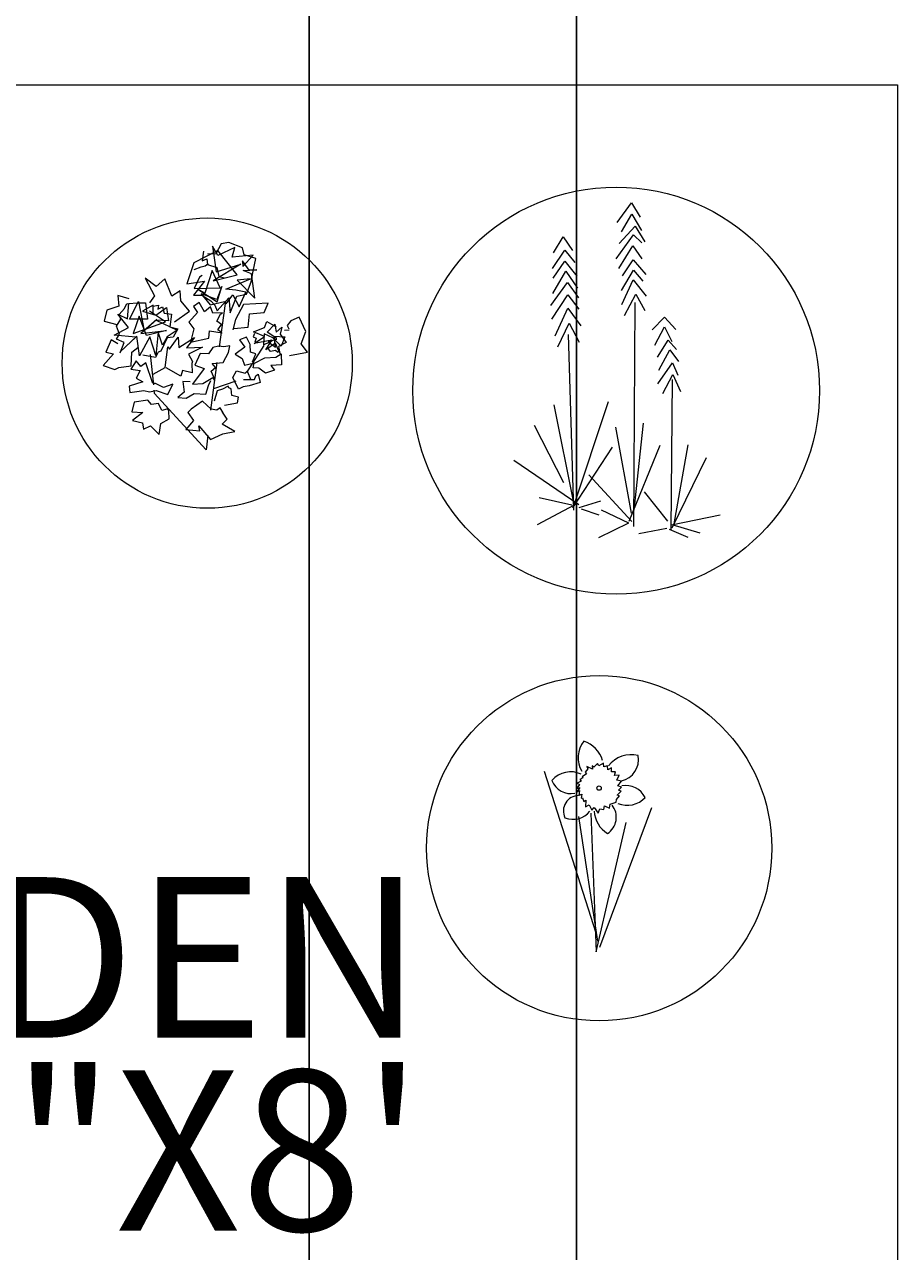
# Model space of a CAD drawing. Units: inches. Extents: x 8049 to 8459, y 820 to 1350.
# Tile 17 of 25: x 8165 to 8197, y 906 to 952. Entities that reach past the tile are written whole.
import ezdxf

# ---------------------------------------------------------------- set-up
doc = ezdxf.new("R2010")
doc.units = ezdxf.units.IN
doc.header["$MEASUREMENT"] = 0
for name, color, linetype, lineweight in [('A-ANNO-DIMS', 2, 'Continuous', 18), ('A-AREA-IDEN', 7, 'Continuous', 25), ('L-PLNT-BEDS', 94, 'Continuous', 18), ('zelen', 69, 'Continuous', 13)]:
    doc.layers.add(name, color=color, linetype=linetype, lineweight=lineweight)
doc.styles.get("Standard").update_dxf_attribs({"font": 'arial.ttf'})
doc.dimstyles.get("Standard").update_dxf_attribs({"dimtxt": 0.18, "dimasz": 0.18, "dimexe": 0.18, "dimexo": 0.0625, "dimgap": 0.09, "dimtad": 0, "dimtih": 1, "dimtoh": 1, "dimdec": 4, "dimzin": 0, "dimdsep": 46, "dimtxsty": 'Standard', "dimcen": 0.09, "dimadec": 0, "dimazin": 0, "dimtfac": 1, "dimtdec": 4, "dimtofl": 0, "dimtmove": 0, "dimatfit": 3, "dimfxl": 1, "dimtolj": 1, "dimtzin": 0, "dimarcsym": 0})

# ---------------------------------------------------------------- blocks, each defined once
blk = doc.blocks.new('z_05')
for p, q in [((36.3, 389.4), (-47, 347)), ((-12.6, 387.1), (-18.2, 353.9)), ((18.3, 405.2), (30.8, 316.1)), ((36.6, 372.7), (18.3, 405.2)), ((47.7, 413.4), (29.2, 377.9)), ((103.3, 306), (36.3, 389.4)), ((74.4, 417.3), (47.7, 413.4)), ((95.8, 400.3), (55.9, 381.9)), ((122.3, 398.9), (74.4, 417.3)), ((86.6, 366.4), (95.8, 400.3)), ((127.9, 375.3), (122.3, 398.9)), ((-47, 347), (-70.6, 274.7)), ((-18.2, 353.9), (-1, 361.5)), ((-6.8, 337.2), (2.7, 345.1)), ((-1, 361.5), (0.6, 341.4)), ((0.6, 341.4), (32.6, 331.6)), ((29.2, 377.9), (0.9, 377.3)), ((116, 342.1), (21, 284.9)), ((30.8, 316.1), (116, 342.1)), ((55.9, 381.9), (36.6, 372.7)), ((158.8, 374.3), (86.6, 366.4)), ((122.6, 354.6), (122.8, 334.2)), ((145.3, 321.4), (122.6, 354.6)), ((122.8, 334.2), (158.8, 374.3)), ((168.1, 362.8), (127.9, 375.3)), ((159.1, 318.4), (168.1, 362.8)), ((-45.7, 324.7), (-21.4, 333.2)), ((-26.7, 298.1), (-45.4, 258.6)), ((-17.9, 303), (-26.7, 298.1)), ((-21.4, 333.2), (-6.8, 337.2)), ((17, 320.7), (-8.1, 242.2)), ((44.8, 260.6), (17, 320.7)), ((21, 284.9), (103.3, 306)), ((32.6, 331.6), (40.3, 300)), ((40.3, 300), (59.6, 295.4)), ((124.7, 321.1), (172, 322.7)), ((153, 309.2), (124.7, 321.1)), ((172, 322.7), (145.3, 321.4)), ((152.5, 282), (159.1, 318.4)), ((164.9, 225.4), (153, 309.2)), ((-214.6, 294.2), (-182.9, 233.1)), ((-176.8, 265.8), (-214.6, 294.2)), ((-147, 291.7), (-176.8, 265.8)), ((-122.2, 232.2), (-147, 291.7)), ((-70.6, 274.7), (-9.7, 283.3)), ((-9.7, 283.3), (-47.6, 235.3)), ((-45.4, 258.6), (44.8, 260.6)), ((-32.2, 256.7), (34.5, 212)), ((-8.1, 242.2), (-32.2, 256.7)), ((50.3, 265.9), (32.6, 220.2)), ((34.5, 212), (50.3, 265.9)), ((63.8, 256.3), (149.6, 291.5)), ((98.5, 252.7), (63.8, 256.3)), ((149.6, 291.5), (103.8, 287.6)), ((103.8, 287.6), (164.9, 225.4)), ((136.1, 238.6), (152.5, 282)), ((-309.5, 234.4), (-305.8, 197.1)), ((-270.2, 222.5), (-309.5, 234.4)), ((-269.3, 152.8), (-238.3, 213.9)), ((-238.3, 213.9), (-219, 112.4)), ((-182.9, 233.1), (-200.1, 208.7)), ((-93.7, 249.9), (-122.2, 232.2)), ((-92, 215.4), (-93.7, 249.9)), ((-61.3, 180), (-92, 215.4)), ((-47.6, 235.3), (-18.5, 235)), ((-20.6, 240.2), (9.6, 201.8)), ((32.6, 220.2), (-20.6, 240.2)), ((-18.5, 235), (12, 215.9)), ((9.6, 201.8), (59.9, 213.6)), ((12, 215.9), (26.8, 200.5)), ((34.5, 180.8), (74.9, 225.8)), ((59.9, 213.6), (65.9, 205.1)), ((65.9, 205.1), (89, 236.9)), ((74.9, 225.8), (79.7, 173.9)), ((79.7, 173.9), (102.7, 232.4)), ((89, 236.9), (110.4, 195.2)), ((133.2, 245.8), (98.5, 252.7)), ((102.7, 232.4), (136.1, 238.6)), ((110.4, 195.2), (133.2, 245.8)), ((-348.1, 183.4), (-357.4, 145.5)), ((-305.8, 197.1), (-348.1, 183.4)), ((-309.5, 169.9), (-275.9, 153.5)), ((-272.4, 123.9), (-309.5, 169.9)), ((-305.7, 168.7), (-286.6, 188.7)), ((-286.6, 188.7), (-279, 206.4)), ((-279, 206.4), (-271.8, 204.4)), ((-275.9, 153.5), (-271.1, 207)), ((-271.1, 207), (-242.8, 209.3)), ((-242.8, 209.3), (-214.2, 208.4)), ((-187.8, 200.8), (-224.5, 180.1)), ((-224.5, 180.1), (-178.5, 166)), ((-214.2, 208.4), (-206.8, 152.2)), ((-144.4, 143), (-200.5, 180.1)), ((-188.9, 197.7), (-168.6, 200.5)), ((-187, 168.3), (-187.8, 200.8)), ((-178.5, 166), (-140.9, 192.9)), ((-168.6, 200.5), (-171.2, 187.4)), ((-171.2, 187.4), (-155.1, 195.5)), ((-155.1, 195.5), (-149.1, 172.6)), ((-149.1, 172.6), (-124.4, 169.6)), ((-140.9, 192.9), (-133.8, 146.3)), ((-113.4, 143.1), (-61.3, 180)), ((-33.6, 175.7), (-64.3, 142.3)), ((-28.6, 209.9), (-48, 196.2)), ((-48, 196.2), (-33.6, 175.7)), ((-10, 177.5), (-28.6, 209.9)), ((10.9, 194.8), (-10, 177.5)), ((19.4, 173.3), (10.9, 194.8)), ((53.3, 173.7), (19.4, 173.3)), ((26.8, 200.5), (34.5, 180.8)), ((42.3, 56.3), (63, 206.2)), ((45.7, 169.6), (53.3, 173.7)), ((125, 202.6), (98, 151)), ((211.1, 208.1), (125, 202.6)), ((141.3, 124.8), (146.2, 170.9)), ((146.2, 170.9), (197.5, 175.4)), ((197.5, 175.4), (211.1, 208.1)), ((-357.4, 145.5), (-313.2, 134.2)), ((-314.6, 127.8), (-299.4, 152.8)), ((-303.6, 100.1), (-314.6, 127.8)), ((-299.4, 152.8), (-305.7, 168.7)), ((-206.8, 152.2), (-269.3, 152.8)), ((-236.2, 163), (-257.1, 102.9)), ((-257.1, 102.9), (-144.4, 143)), ((-210, 96), (-236.2, 163)), ((-174.3, 151.5), (-230.4, 103.2)), ((-219, 112.4), (-174.3, 151.5)), ((-177.2, 148.6), (-104.7, 113.7)), ((-133.8, 146.3), (-177.2, 148.6)), ((-124.4, 169.6), (-129.3, 125.2)), ((-64.3, 142.3), (-46.8, 118.9)), ((33.2, 145.5), (45.7, 169.6)), ((49.2, 133.6), (33.2, 145.5)), ((36.7, 115.6), (49.2, 133.6)), ((98, 151), (88.7, 115.9)), ((198.5, 123.6), (206.2, 144.3)), ((206.2, 144.3), (238.2, 125.2)), ((207.2, 107.5), (234.5, 134.4)), ((234.5, 134.4), (238.7, 107.5)), ((289, 146.8), (276.7, 130.9)), ((276.7, 130.9), (282.3, 119)), ((318.2, 159), (289, 146.8)), ((341.6, 110.1), (318.2, 159)), ((-322.2, 96.6), (-272.4, 123.9)), ((-247, 90.1), (-322.2, 96.6)), ((-314.4, 82.9), (-303.6, 100.1)), ((-244.4, 93.4), (-301.8, 39.5)), ((-301.8, 39.5), (-247, 90.1)), ((-234.9, 25.3), (-244.4, 93.4)), ((-199.4, 90.7), (-234.9, 25.3)), ((-230.4, 103.2), (-141.2, 113.4)), ((-141.2, 113.4), (-210, 96)), ((-177.7, 26.3), (-199.4, 90.7)), ((-170.3, 107.2), (-177.7, 26.3)), ((-154.7, 62.5), (-170.3, 107.2)), ((-138.6, 87.7), (-161.1, 41.4)), ((-138.8, 91.1), (-154.7, 62.5)), ((-104.7, 113.7), (-138.8, 91.1)), ((-117.9, 89.5), (-138.6, 87.7)), ((-130.7, 48.4), (-100.9, 90.4)), ((-129.3, 125.2), (-102.3, 118.9)), ((-102.3, 118.9), (-117.9, 89.5)), ((-100.9, 90.4), (-98.5, 54.7)), ((-98.5, 54.7), (-43.7, 88.9)), ((-43.7, 88.9), (-71.8, 53.1)), ((-46.8, 118.9), (-58.1, 72.1)), ((-58.1, 72.1), (5.6, 86.3)), ((5.6, 86.3), (7.6, 111.7)), ((7.6, 111.7), (51.8, 105.2)), ((48.6, 107.6), (36.7, 115.6)), ((91.6, 119.6), (141.3, 124.8)), ((135.5, 89.5), (111.9, 81.1)), ((148.3, 64.3), (135.5, 89.5)), ((163.2, 102.8), (159.3, 91.6)), ((159.3, 91.6), (169, 86.6)), ((159.9, 108.8), (198.5, 123.6)), ((197.7, 92.7), (159.9, 108.8)), ((162.5, 68.1), (197.7, 92.7)), ((169, 86.6), (165, 72.9)), ((196.9, 101.2), (195.1, 63.5)), ((226.8, 87.8), (196.9, 101.2)), ((241.1, 84.8), (207.2, 107.5)), ((255.9, 59.2), (226.8, 87.8)), ((231.3, 94), (268.9, 91.4)), ((236.9, 55.9), (231.3, 94)), ((238.7, 107.5), (258, 124.6)), ((258, 124.6), (252.2, 100.6)), ((252.2, 100.6), (273.6, 71.3)), ((268.9, 91.4), (255.9, 59.2)), ((284.1, 114.7), (267.1, 113.5)), ((324.9, 66.8), (341.6, 110.1)), ((-333.3, 80.8), (-351, 37.5)), ((-309.7, 66.5), (-333.3, 80.8)), ((-288, 71.4), (-314.4, 82.9)), ((-302, 35.3), (-288, 71.4)), ((-260.8, 38.4), (-240.2, 53.7)), ((-145.9, -14.9), (-136.6, 56.2)), ((-136.6, 56.2), (-130.7, 48.4)), ((-71.8, 53.1), (-16.6, 55.1)), ((-16.6, 55.1), (-64.6, 31.5)), ((19, 54.4), (4.5, 32.1)), ((38.8, 58.6), (19, 54.4)), ((57.8, 57), (38.8, 58.6)), ((78.7, 59.7), (57.8, 57)), ((73.6, 37.4), (78.7, 59.7)), ((130.2, 55.1), (97.1, 31.2)), ((111.9, 81.1), (130.2, 55.1)), ((137.3, -32.7), (196.8, 60.8)), ((149.9, 38.3), (148.3, 64.3)), ((223.6, 79.6), (162.5, 68.1)), ((195.1, 63.5), (241.1, 84.8)), ((203.3, 46.4), (223.6, 79.6)), ((236.3, 69.4), (203.3, 46.4)), ((239.5, 81.5), (211.5, 73.6)), ((211.5, 73.6), (236.9, 55.9)), ((218.6, 40.3), (212.6, 49.9)), ((236.5, 44), (218.6, 40.3)), ((250.9, 32.9), (236.3, 69.4)), ((244.2, 36.6), (236.5, 44)), ((273.6, 71.3), (246.7, 57.2)), ((246.7, 57.2), (250.9, 32.9)), ((347.5, 37.8), (324.9, 66.8)), ((-324.2, 32.6), (-360.1, -8.6)), ((-351, 37.5), (-324.2, 32.6)), ((-246.1, 8.6), (-264.6, -20.3)), ((-263.3, -9.2), (-260.8, 38.4)), ((-229.7, -11.4), (-246.1, 8.6)), ((-212.5, 1.1), (-229.7, -11.4)), ((-179.1, 19.6), (-222.6, 27.6)), ((-188.1, -70.9), (-212.5, 1.1)), ((-197.6, 30.4), (-186.7, -75.1)), ((-170.2, 37.7), (-179.1, 19.6)), ((-161.1, 41.4), (-170.2, 37.7)), ((-64.6, 31.5), (-51.4, 5.7)), ((-51.4, 5.7), (-53.3, -1)), ((-24.4, 33.3), (-43.1, -6.5)), ((4.5, 32.1), (-24.4, 33.3)), ((12.2, -162.5), (34.8, 2)), ((17.3, -0.7), (54.6, 2.8)), ((54.6, 2.8), (73.6, 37.4)), ((97.1, 31.2), (121.2, 16.7)), ((121.2, 16.7), (128.5, -6.7)), ((168.1, 32.5), (149.9, 38.3)), ((156.5, 4.8), (168.1, 32.5)), ((159.5, -16), (162.4, 0.9)), ((163.5, 0), (199.5, 18.3)), ((199.5, 18.3), (237.6, 20.3)), ((237.6, 20.3), (256.2, 32.8)), ((256.2, 32.8), (257.4, -5.3)), ((284.6, 26.2), (347.5, 37.8)), ((-360.1, -8.6), (-319.8, -21.4)), ((-319.8, -21.4), (-305.8, -15)), ((-305.8, -15), (-263.3, -9.2)), ((-264.6, -20.3), (-232.2, -25.5)), ((-232.2, -25.5), (-245.8, -51.9)), ((-187.7, -38.6), (-145.9, -14.9)), ((-91.7, -44.5), (-142, -16)), ((-85.5, -25.9), (-91.7, -44.5)), ((-52.3, -34), (-85.5, -25.9)), ((-53.3, -1), (-52.3, -34)), ((-11.2, -18.3), (-50.9, -72.3)), ((-43.1, -6.5), (-11.2, -18.3)), ((14.1, -27.4), (28.8, -14.9)), ((25.9, -56.8), (14.1, -27.4)), ((28.8, -14.9), (17.3, -0.7)), ((88.3, -50.2), (101.1, -26.2)), ((101.1, -26.2), (131.6, -34.3)), ((128.5, -6.7), (158.7, -0.6)), ((131.6, -34.3), (137.9, -27.4)), ((137.9, -27.4), (150.4, -57.2)), ((179.2, -17.2), (159.5, -16)), ((168.4, -43.5), (176.2, -37.8)), ((176.2, -37.8), (183.5, -67.3)), ((201.2, -35.1), (179.2, -17.2)), ((232.4, -24.4), (201.2, -35.1)), ((257.4, -5.3), (219.7, -8.5)), ((219.7, -8.5), (232.4, -24.4)), ((-222.9, -64.1), (-270.2, -79.3)), ((-270.2, -79.3), (-268.3, -101.3)), ((-245.8, -51.9), (-222.9, -64.1)), ((-179.4, -70.6), (-185, -70.2)), ((-151.1, -84.7), (-179.4, -70.6)), ((-119.1, -72.9), (-151.1, -84.7)), ((-137, -108.6), (-119.1, -72.9)), ((-84.6, -63.8), (-80.4, -99.9)), ((-59, -65.1), (-84.6, -63.8)), ((-50.9, -72.3), (-15.2, -70.2)), ((-15.2, -70.2), (19.4, -49.1)), ((-5.1, -107.6), (3.9, -77.8)), ((3.9, -77.8), (12.1, -59.8)), ((19.4, -49.1), (24.6, -59.5)), ((99.1, -62.5), (22.1, -89.1)), ((72.1, -79.9), (52.8, -90)), ((75, -85.4), (72.1, -79.9)), ((107.8, -89.9), (88.3, -50.2)), ((124.2, -82.4), (107.8, -89.9)), ((123.4, -54.1), (123.7, -54)), ((145.4, -78.6), (124.2, -82.4)), ((125.8, -57.1), (163.6, -56.6)), ((183.5, -67.3), (145.4, -78.6)), ((163.6, -56.6), (168.4, -43.5)), ((-268.3, -101.3), (-219.9, -94.9)), ((-219.9, -94.9), (-199.8, -99.2)), ((-199.8, -99.2), (-177.4, -94.6)), ((-184.9, -93), (-183.8, -103.6)), ((-183.8, -103.6), (-3.6, -299.6)), ((-177.4, -94.6), (-137, -108.6)), ((-80.4, -99.9), (-101.4, -118.3)), ((-101.4, -118.3), (-72.6, -121.5)), ((-72.6, -121.5), (-45.6, -105.4)), ((-45.6, -105.4), (-5.1, -107.6)), ((34.7, -95.4), (23.5, -131.1)), ((52.8, -90), (34.7, -95.4)), ((82.5, -89.1), (75, -85.4)), ((85.1, -112.3), (82.5, -89.1)), ((108, -117.3), (85.1, -112.3)), ((104.9, -137.2), (108, -117.3)), ((-253.7, -134.6), (-261.4, -168.3)), ((-261.4, -168.3), (-223.5, -170.8)), ((-205.8, -128), (-253.7, -134.6)), ((-192.7, -142.7), (-205.8, -128)), ((-168.7, -140.1), (-192.7, -142.7)), ((-157, -164.4), (-168.7, -140.1)), ((-139.9, -158.9), (-157, -164.4)), ((-133.5, -165.3), (-138.4, -154.1)), ((-131.8, -192.3), (-133.5, -165.3)), ((-55.5, -159.5), (-67.8, -171.1)), ((-16.2, -131.7), (-55.5, -159.5)), ((13.1, -159.3), (-16.2, -131.7)), ((32.6, -162.8), (13.1, -159.3)), ((45, -154.1), (32.6, -162.8)), ((55.2, -172.3), (45, -154.1)), ((69.1, -193.4), (52.3, -169.2)), ((59.4, -145.7), (104.9, -137.2)), ((-223.5, -170.8), (-259.2, -198.1)), ((-259.2, -198.1), (-224.7, -206)), ((-224.7, -206), (-221.4, -228.1)), ((-166.3, -247.2), (-160.4, -209.4)), ((-160.4, -209.4), (-131.8, -192.3)), ((-47.6, -198.1), (-74.3, -229.2)), ((-67.8, -171.1), (-47.6, -198.1)), ((51.3, -211.7), (69.1, -193.4)), ((95.2, -236.2), (51.3, -211.7)), ((-221.4, -228.1), (-196.4, -217.5)), ((-196.4, -217.5), (-166.3, -247.2)), ((-74.3, -229.2), (-25.6, -233.9)), ((-29.7, -216.4), (11.5, -264)), ((-25.6, -233.9), (-29.7, -216.4)), ((2.5, -250.9), (-3.6, -299.6)), ((11.5, -264), (54, -244.9)), ((54, -244.9), (95.2, -236.2))]:
    blk.add_line(p, q)
blk.add_circle((0, 0), 502.5)
blk = doc.blocks.new('z_04')
for p, q in [((2.7, 414.9), (37.8, 463.9)), ((37.8, 463.9), (59.6, 428.2)), ((13.1, 392), (38.9, 435.6)), ((38.9, 435.6), (62.3, 395.4)), ((7.3, 362.9), (46.8, 406.2)), ((46.8, 406.2), (71, 367.7)), ((-154.8, 340), (-131.1, 379.6)), ((-131.1, 379.6), (-108, 346.2)), ((0, 325.8), (42.4, 384.4)), ((42.4, 384.4), (63.1, 364.6)), ((-157.2, 301.5), (-126.5, 346.8)), ((-126.5, 346.8), (-102.5, 316.5)), ((6.3, 301.8), (40.8, 357.5)), ((40.8, 357.5), (63.6, 325.5)), ((-155.9, 278), (-126.5, 319.9)), ((-126.5, 319.9), (-97.4, 282.8)), ((15.2, 283.7), (41.9, 323.3)), ((41.9, 323.3), (72.9, 287.1)), ((-156.9, 239.8), (-124.6, 295)), ((-124.6, 295), (-95.5, 253.1)), ((12.8, 247.5), (42.7, 297.5)), ((13.9, 213), (42.2, 273.2)), ((42.2, 273.2), (73.7, 233.6)), ((42.7, 297.5), (66.1, 270.4)), ((-161.6, 209.9), (-120.2, 267)), ((-120.2, 267), (-93.3, 229.4)), ((-159.1, 176.8), (-119.4, 236.5)), ((-119.4, 236.5), (-92.5, 201.1)), ((20.4, 185.3), (48.4, 238.1)), ((43.8, -335.7), (46.5, 217.8)), ((48.4, 238.1), (70.4, 198)), ((-150.7, 134.9), (-119.7, 203.9)), ((-119.7, 203.9), (-87.6, 159.8)), ((-144.4, 107.8), (-116.4, 166.9)), ((-116.4, 166.9), (-91.4, 119.9)), ((89.2, 150.5), (119.4, 181.3)), ((95.5, 112), (119.1, 157.3)), ((119.1, 157.3), (137.6, 121.6)), ((119.4, 181.3), (147.7, 150.8)), ((-104.4, -294.9), (-117.5, 138.6)), ((102, 82.9), (128.4, 124.4)), ((128.4, 124.4), (149.3, 101.5)), ((105, 50.3), (132.7, 100.7)), ((132.7, 100.7), (153.7, 71.6)), ((102.5, 16.7), (138.7, 68.7)), ((138.7, 68.7), (152.6, 38.5)), ((115.6, -6.8), (140.1, 40.2)), ((140.1, 40.2), (159.1, -2)), ((136, -344.8), (139.5, 27.2)), ((-106.6, -289.6), (-19.3, -26.6)), ((-105, -276.9), (-153.1, -35.1)), ((-129.5, -227.7), (-202.1, -86.3)), ((38.1, -302.9), (-0.8, -90.5)), ((44.1, -294.7), (67.5, -80)), ((-107.2, -289.3), (-9.5, -139.2)), ((32.4, -322.2), (108.5, -134.3)), ((143.3, -329.2), (178.2, -133.5)), ((-92.5, -282), (-253, -172.8)), ((138.4, -339.1), (223, -165.2)), ((38.9, -322.7), (-67.2, -207.9)), ((-109.3, -282.6), (-190.4, -264.7)), ((-91.1, -288.8), (-37.8, -272.1)), ((127.8, -321.9), (69.9, -249.5)), ((-104.2, -282.8), (-195, -331.5)), ((-86.5, -292.2), (-42.7, -306.9)), ((31, -327.5), (-36.2, -295)), ((30.5, -327.5), (-44.1, -363.4)), ((136.8, -330.9), (256.5, -306.9)), ((137.1, -330.6), (207, -351.3)), ((125.4, -340), (56.3, -353.3)), ((131.1, -341.7), (177.3, -361.8))]:
    blk.add_line(p, q)
blk.add_circle((0, 0), 502.5)
blk = doc.blocks.new('z_08')
for p, q in [((-8.4, -246.7), (-159.3, 223.2)), ((1.5, -287.6), (152.7, 118.6)), ((-4.2, -270.1), (-58.8, 92)), ((-24, 101.7), (-8.7, -301.4)), ((-8.7, -301.4), (78.6, 74.5))]:
    blk.add_line(p, q)
blk.add_lwpolyline([(-36.3, 236.9), (-32.6, 230.3), (-41.2, 220.4), (-36.5, 216.2), (-49.7, 207), (-47.3, 203.9), (-56.6, 199.7), (-52.3, 194.9), (-63.8, 188.8), (-57.4, 185.2), (-65.8, 172.2), (-56.3, 176), (-64.1, 164.1), (-57, 167.5), (-59.7, 153), (-57.8, 153.7), (-50.7, 157.1), (-52.8, 145.2), (-48.1, 146.5), (-45, 135.3), (-38.5, 139.3), (-40.2, 120.4), (-28.8, 125.8), (-21.2, 110.3), (-14.4, 117.9), (-3.3, 101.4), (2, 114.8), (13.5, 112.2), (15.1, 122.7), (29.6, 116.1), (31.8, 127.6), (49.7, 133.8), (50.1, 141.4), (58.8, 151.7), (52.1, 153.6), (64.2, 165.2), (56.2, 168.6), (64.4, 177.6), (53.7, 181.6), (64.6, 194.7), (51.7, 197.5), (58.1, 211.7), (44.3, 211.1), (47, 222), (36.1, 222), (35.4, 233.6), (25.1, 227.9), (23.8, 239.3), (13.1, 236.2), (12.5, 246.7), (-1.1, 239.3), (-4.7, 246.4), (-15.5, 235.7), (-20.6, 239.4), (-19.7, 229.8), (-36.3, 236.9)])
for centre, radius in [((0, 0), 501.6), ((-0.3, 174.4), 6.32)]:
    blk.add_circle(centre, radius)
for centre, radius, start, end in [((18.1, 262.8), 79.4, 142.6945, 209.6234), ((-71.1, 230.6), 84.5, 16.4392, 72.0686), ((92.3, 189.3), 82.4, 75.3361, 142.797), ((51, 257.3), 63.3, 282.6991, 10.6878), ((-83.4, 151.9), 70, 63.8597, 140.3167), ((-82.2, 217.5), 58.9, 200.8344, 281.4173), ((76.9, 117.5), 64.4, 27.9746, 99.6629), ((-59.4, 108.2), 44.7, 90.8466, 206.078), ((81.2, 195.8), 71.2, 247.7997, 317.4677), ((-75.6, 144.7), 61, 246.9504, 322.7891), ((70, 113.9), 85.1, 184.0633, 237.2607), ((-7.1, 90), 56.9, 303.1089, 38.3983)]:
    blk.add_arc(centre, radius, start, end)
blk = doc.blocks.new('*D58')
at = {"layer": 'A-ANNO-DIMS', "color": 0, "lineweight": -2, "transparency": 16777216}
for p, q in [((8139.397, 1162.808), (8139.397, 820.091)), ((8175.397, 1162.808), (8175.397, 820.091)), ((8139.577, 820.271), (8157.179, 820.271)), ((8175.217, 820.271), (8157.616, 820.271))]:
    blk.add_line(p, q, dxfattribs=at)
at = {"layer": 'A-ANNO-DIMS', "color": 0, "transparency": 16777216}
for points in [[(8139.577, 820.301), (8139.577, 820.241), (8139.397, 820.271)], [(8175.217, 820.301), (8175.217, 820.241), (8175.397, 820.271)]]:
    blk.add_solid(points, dxfattribs=at)
at = {"layer": 'Defpoints', "color": 0, "transparency": 16777216}
for p in [(8139.397, 1162.871), (8175.397, 1162.871), (8175.397, 820.271)]:
    blk.add_point(p, dxfattribs=at)
at = {"layer": 'A-ANNO-DIMS', "color": 0, "transparency": 16777216, "insert": (8157.397, 820.271), "char_height": 0.18, "attachment_point": 5}
blk.add_mtext('\\A1;36', dxfattribs=at)
blk = doc.blocks.new('*D71')
at = {"layer": 'A-ANNO-DIMS', "color": 0, "lineweight": -2, "transparency": 16777216}
for p, q in [((8185.397, 1045.808), (8185.397, 820.091)), ((8239.397, 1045.808), (8239.397, 820.091)), ((8185.577, 820.271), (8212.179, 820.271)), ((8239.217, 820.271), (8212.616, 820.271))]:
    blk.add_line(p, q, dxfattribs=at)
at = {"layer": 'A-ANNO-DIMS', "color": 0, "transparency": 16777216}
for points in [[(8185.577, 820.301), (8185.577, 820.241), (8185.397, 820.271)], [(8239.217, 820.301), (8239.217, 820.241), (8239.397, 820.271)]]:
    blk.add_solid(points, dxfattribs=at)
at = {"layer": 'Defpoints', "color": 0, "transparency": 16777216}
for p in [(8185.397, 1045.871), (8239.397, 1045.871), (8239.397, 820.271)]:
    blk.add_point(p, dxfattribs=at)
at = {"layer": 'A-ANNO-DIMS', "color": 0, "transparency": 16777216, "insert": (8212.397, 820.271), "char_height": 0.18, "attachment_point": 5}
blk.add_mtext('\\A1;54', dxfattribs=at)
blk = doc.blocks.new('*D76')
at = {"layer": 'A-ANNO-DIMS', "color": 0, "lineweight": -2, "transparency": 16777216}
for p, q in [((8083.397, 1054.808), (8083.397, 820.091)), ((8299.397, 1054.808), (8299.397, 820.091)), ((8083.577, 820.271), (8191.107, 820.271)), ((8299.217, 820.271), (8191.688, 820.271))]:
    blk.add_line(p, q, dxfattribs=at)
at = {"layer": 'A-ANNO-DIMS', "color": 0, "transparency": 16777216}
for points in [[(8083.577, 820.301), (8083.577, 820.241), (8083.397, 820.271)], [(8299.217, 820.301), (8299.217, 820.241), (8299.397, 820.271)]]:
    blk.add_solid(points, dxfattribs=at)
at = {"layer": 'Defpoints', "color": 0, "transparency": 16777216}
for p in [(8083.397, 1054.871), (8299.397, 1054.871), (8299.397, 820.271)]:
    blk.add_point(p, dxfattribs=at)
at = {"layer": 'A-ANNO-DIMS', "color": 0, "transparency": 16777216, "insert": (8191.397, 820.271), "char_height": 0.18, "attachment_point": 5}
blk.add_mtext('\\A1;216', dxfattribs=at)

msp = doc.modelspace()

# ---------------------------------------------------------------- linework, layer by layer
at = {"layer": 'L-PLNT-BEDS'}
for p, q in [((8083.3974, 949.8706), (8197.3974, 949.8706)), ((8197.3974, 949.8706), (8197.3974, 853.8706))]:
    msp.add_line(p, q, dxfattribs=at)

# ---------------------------------------------------------------- block references
at = {"layer": 'zelen'}
for name, p, xscale, yscale, zscale in [('z_04', (8186.8786, 938.4475), 0.0151365556588967, 0.0151365556588967, 0.0151365556588967), ('z_05', (8171.5864, 939.4743), 0.0107957317921007, 0.0107957317921007, 0.0107957317921007), ('z_08', (8186.2436, 921.3488), 0.0128650146468131, 0.0128650146468131, 0.0128650146468131)]:
    msp.add_blockref(name, p, dxfattribs=dict(at, xscale=xscale, yscale=yscale, zscale=zscale))

# ---------------------------------------------------------------- texts
at = {"layer": 'A-AREA-IDEN'}
for s, p in [('GARDEN', (8147.4444, 914.2666)), ('9\'6"X8\'', (8152.9088, 907.0536))]:
    msp.add_text(s, height=6, dxfattribs=at).set_placement(p)

# ---------------------------------------------------------------- dimensions: what is measured, and where the dimension line sits
at = {"layer": 'A-ANNO-DIMS'}
for base, p1, p2, picture, middle in [((8175.3974, 820.2706), (8139.3974, 1162.8706), (8175.3974, 1162.8706), '*D58', (8157.3974, 820.2706)), ((8299.3974, 820.2706), (8083.3974, 1054.8706), (8299.3974, 1054.8706), '*D76', (8191.3974, 820.2706)), ((8239.3974, 820.2706), (8185.3974, 1045.8706), (8239.3974, 1045.8706), '*D71', (8212.3974, 820.2706))]:
    dim = msp.add_linear_dim(base=base, p1=p1, p2=p2, dimstyle='Standard', override={"dimdec": 0, "dimlfac": 1, "dimrnd": 0, "dimzin": 0, "dimdsep": 46, "dimlunit": 2}, dxfattribs=at)
    dim.commit()
    dim.dimension.update_dxf_attribs({"geometry": picture, "text_midpoint": middle})

doc.saveas('drawing.dxf')
